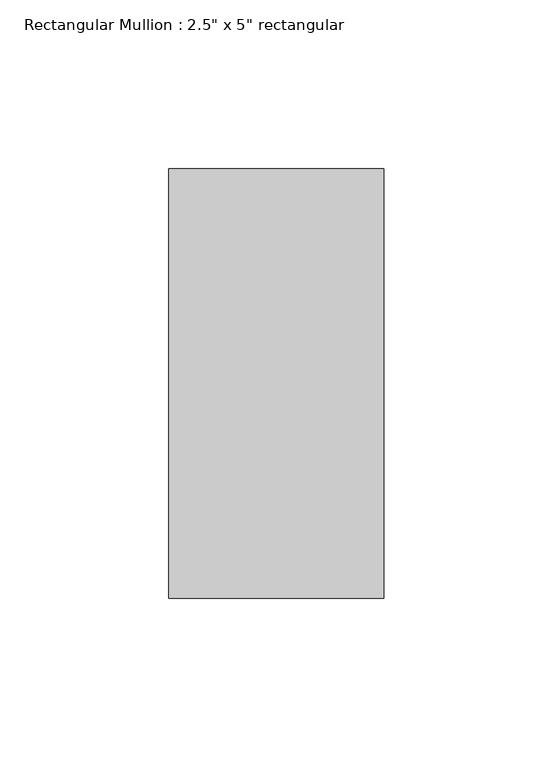
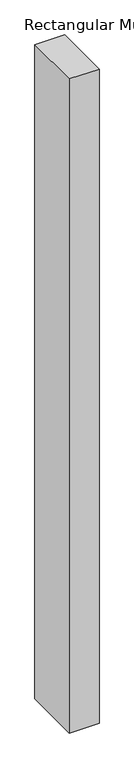
"""IFC4 building model written with IfcOpenShell, lengths in millimetres: member geometry."""

from ifc_helpers import new_model, si_unit, frame, origin, place, context, project, spatial, polyline, outline, extrude, source, transform, mapped, element, save


def member_673fd8de(model_context):
    return source(origin(), model_context, "Body", "SweptSolid", [
        extrude(outline(polyline([(31.75, 63.5), (31.75, -63.5), (-31.75, -63.5), (-31.75, 63.5), (31.75, 63.5)])), frame((0.0, 0.0, -1475.8013618), z_axis=(0.0, 0.0, 1.0), x_axis=(1.0, 0.0, 0.0)), (0.0, 0.0, 1.0), 1475.8013618),
    ])


if __name__ == "__main__":
    model = new_model("IFC4")
    model_context = context("Model", 3, world=origin())
    ifc_project = project(units=[si_unit("LENGTHUNIT", "METRE", prefix="MILLI")], contexts=[model_context])
    site = spatial("IfcSite", under=ifc_project)
    building = spatial("IfcBuilding", under=site)
    placement = place(None, origin())
    member_shape = member_673fd8de(model_context)
    element("IfcMember", 1, ObjectType="Rectangular Mullion : 2.5\" x 5\" rectangular", at=placement, inside=building, context=model_context, shape_type="MappedRepresentation", body=[
        mapped(member_shape, transform((0.0, 0.0, 0.0), x_axis=(1.0, 0.0, 0.0), y_axis=(0.0, 1.0, 0.0), z_axis=(0.0, 0.0, 1.0))),
    ])
    save(model, "model.ifc")

# Revit data of these elements
# Type "Rectangular Mullion : 2.5\" x 5\" rectangular"
#   built-in parameter 1007304 = 0.416667 (stored number, unit not read)
#   built-in parameter 1007301 = 0.104167 (stored number, unit not read)
#   built-in parameter 1007300 = 0.104167 (stored number, unit not read)
# Element 1 (IfcMember, "Rectangular Mullion : 2.5\" x 5\" rectangular")
#   Materials on its faces: "Aluminum"
# Materials
#   "Aluminum": class "Metal", colour RGB 247 247 247, transparency 0, Description = "Aluminum 6061", Cost = 0
